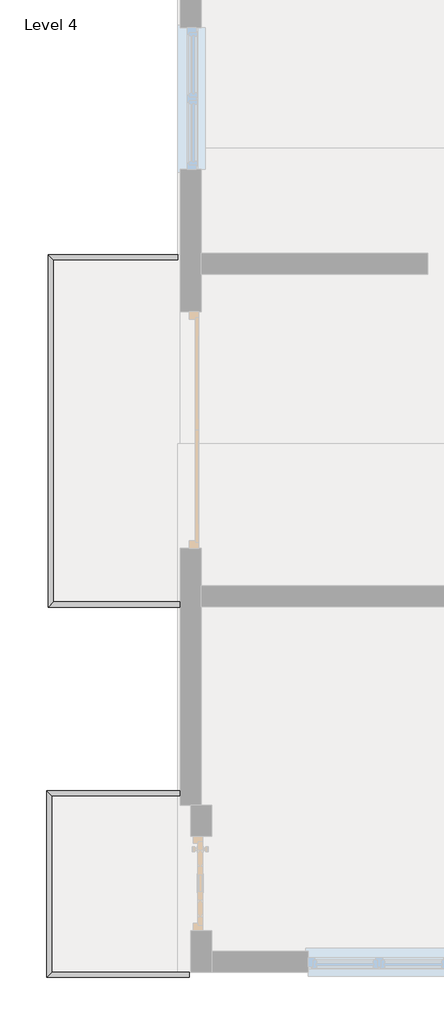
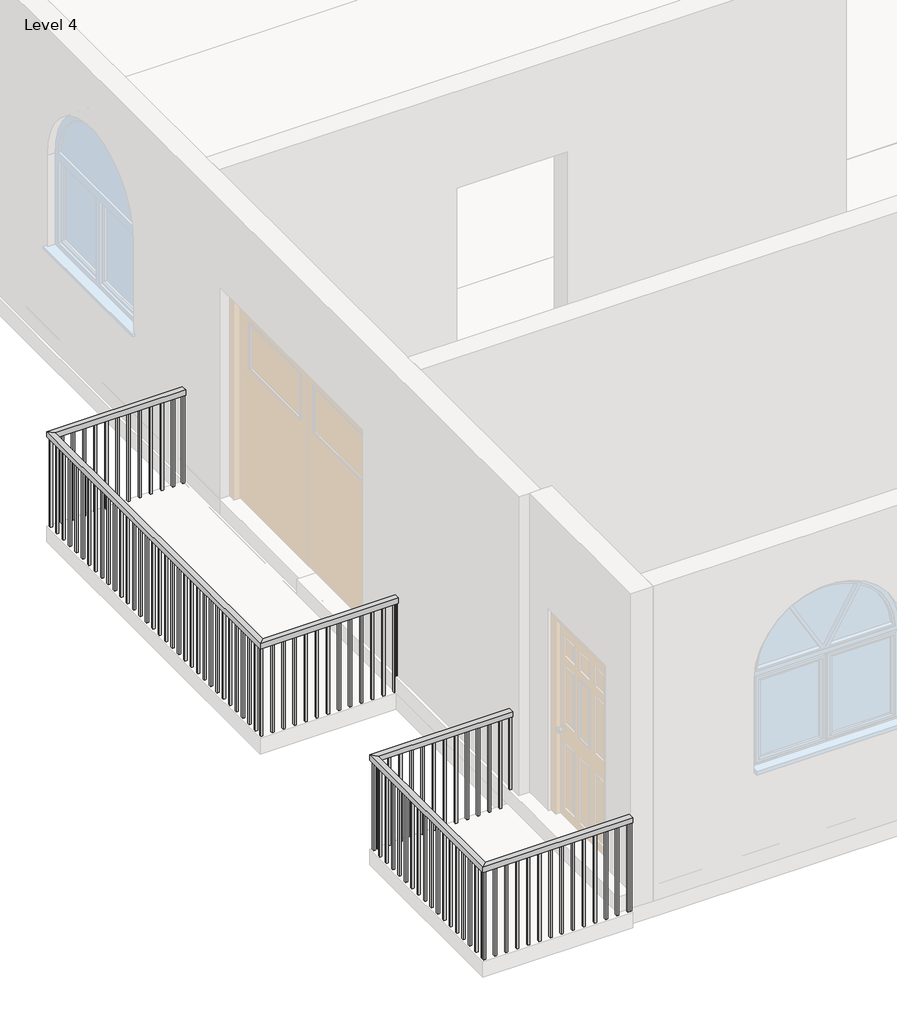
# One storey, part 3 of 7: 2 railings.
"""IFC4 building model written with IfcOpenShell, lengths in millimetres."""

from ifc_helpers import new_model, si_unit, frame, origin, place, context, project, spatial, polyline, outline, extrude, faceted_brep, element, save

model = new_model("IFC4")

# Units and contexts
model_context = context("Model", 3, world=origin())
ifc_project = project(units=[si_unit("LENGTHUNIT", "METRE", prefix="MILLI")], contexts=[model_context])

# Site, building, storey
site = spatial("IfcSite", under=ifc_project)
building = spatial("IfcBuilding", under=site)
storey = spatial("IfcBuildingStorey", under=building, Name="Level 4", Elevation=9144.0)

# Railings
placement = place(None, origin())
element("IfcRailing", 1, ObjectType="Handrail - Rectangular", at=placement, inside=storey, context=model_context, shape_type="SolidModel", body=[
    faceted_brep([(-6354.2109037, -3767.6037749, 10058.4), (-6354.2109037, -3767.6037749, 10007.6), (-6354.2109037, -3716.8037749, 10007.6), (-6354.2109037, -3716.8037749, 10058.4), (-7548.0109037, -3767.6037749, 10058.4), (-7548.0109037, -3767.6037749, 10007.6), (-7598.8109037, -3716.8037749, 10007.6), (-7598.8109037, -3716.8037749, 10058.4), (-7548.0109037, -7054.4894702, 10058.4), (-7548.0109037, -7054.4894702, 10007.6), (-7598.8109037, -7105.2894702, 10007.6), (-7598.8109037, -7105.2894702, 10058.4), (-6330.8013636, -7054.4894702, 10058.4), (-6330.8013636, -7105.2894702, 10058.4), (-6330.8013636, -7105.2894702, 10007.6), (-6330.8013636, -7054.4894702, 10007.6)], [[[0, 1, 2, 3]], [[1, 0, 4, 5]], [[2, 1, 5, 6]], [[3, 2, 6, 7]], [[0, 3, 7, 4]], [[5, 4, 8, 9]], [[6, 5, 9, 10]], [[7, 6, 10, 11]], [[4, 7, 11, 8]], [[12, 13, 14, 15]], [[9, 8, 12, 15]], [[10, 9, 15, 14]], [[11, 10, 14, 13]], [[8, 11, 13, 12]]]),
    extrude(outline(polyline([(-6363.7359037, -7089.4144702), (-6363.7359037, -7070.3644702), (-6344.6859037, -7070.3644702), (-6344.6859037, -7089.4144702), (-6363.7359037, -7089.4144702)])), frame((0.0, 0.0, 9144.0), z_axis=(0.0, 0.0, 1.0), x_axis=(1.0, 0.0, 0.0)), (0.0, 0.0, 1.0), 863.6),
    extrude(outline(polyline([(-6465.3359037, -7089.4144702), (-6465.3359037, -7070.3644702), (-6446.2859037, -7070.3644702), (-6446.2859037, -7089.4144702), (-6465.3359037, -7089.4144702)])), frame((0.0, 0.0, 9144.0), z_axis=(0.0, 0.0, 1.0), x_axis=(1.0, 0.0, 0.0)), (0.0, 0.0, 1.0), 863.6),
    extrude(outline(polyline([(-6566.9359037, -7089.4144702), (-6566.9359037, -7070.3644702), (-6547.8859037, -7070.3644702), (-6547.8859037, -7089.4144702), (-6566.9359037, -7089.4144702)])), frame((0.0, 0.0, 9144.0), z_axis=(0.0, 0.0, 1.0), x_axis=(1.0, 0.0, 0.0)), (0.0, 0.0, 1.0), 863.6),
    extrude(outline(polyline([(-6668.5359037, -7089.4144702), (-6668.5359037, -7070.3644702), (-6649.4859037, -7070.3644702), (-6649.4859037, -7089.4144702), (-6668.5359037, -7089.4144702)])), frame((0.0, 0.0, 9144.0), z_axis=(0.0, 0.0, 1.0), x_axis=(1.0, 0.0, 0.0)), (0.0, 0.0, 1.0), 863.6),
    extrude(outline(polyline([(-6770.1359037, -7089.4144702), (-6770.1359037, -7070.3644702), (-6751.0859037, -7070.3644702), (-6751.0859037, -7089.4144702), (-6770.1359037, -7089.4144702)])), frame((0.0, 0.0, 9144.0), z_axis=(0.0, 0.0, 1.0), x_axis=(1.0, 0.0, 0.0)), (0.0, 0.0, 1.0), 863.6),
    extrude(outline(polyline([(-6871.7359037, -7089.4144702), (-6871.7359037, -7070.3644702), (-6852.6859037, -7070.3644702), (-6852.6859037, -7089.4144702), (-6871.7359037, -7089.4144702)])), frame((0.0, 0.0, 9144.0), z_axis=(0.0, 0.0, 1.0), x_axis=(1.0, 0.0, 0.0)), (0.0, 0.0, 1.0), 863.6),
    extrude(outline(polyline([(-6973.3359037, -7089.4144702), (-6973.3359037, -7070.3644702), (-6954.2859037, -7070.3644702), (-6954.2859037, -7089.4144702), (-6973.3359037, -7089.4144702)])), frame((0.0, 0.0, 9144.0), z_axis=(0.0, 0.0, 1.0), x_axis=(1.0, 0.0, 0.0)), (0.0, 0.0, 1.0), 863.6),
    extrude(outline(polyline([(-7074.9359037, -7089.4144702), (-7074.9359037, -7070.3644702), (-7055.8859037, -7070.3644702), (-7055.8859037, -7089.4144702), (-7074.9359037, -7089.4144702)])), frame((0.0, 0.0, 9144.0), z_axis=(0.0, 0.0, 1.0), x_axis=(1.0, 0.0, 0.0)), (0.0, 0.0, 1.0), 863.6),
    extrude(outline(polyline([(-7176.5359037, -7089.4144702), (-7176.5359037, -7070.3644702), (-7157.4859037, -7070.3644702), (-7157.4859037, -7089.4144702), (-7176.5359037, -7089.4144702)])), frame((0.0, 0.0, 9144.0), z_axis=(0.0, 0.0, 1.0), x_axis=(1.0, 0.0, 0.0)), (0.0, 0.0, 1.0), 863.6),
    extrude(outline(polyline([(-7278.1359037, -7089.4144702), (-7278.1359037, -7070.3644702), (-7259.0859037, -7070.3644702), (-7259.0859037, -7089.4144702), (-7278.1359037, -7089.4144702)])), frame((0.0, 0.0, 9144.0), z_axis=(0.0, 0.0, 1.0), x_axis=(1.0, 0.0, 0.0)), (0.0, 0.0, 1.0), 863.6),
    extrude(outline(polyline([(-7379.7359037, -7089.4144702), (-7379.7359037, -7070.3644702), (-7360.6859037, -7070.3644702), (-7360.6859037, -7089.4144702), (-7379.7359037, -7089.4144702)])), frame((0.0, 0.0, 9144.0), z_axis=(0.0, 0.0, 1.0), x_axis=(1.0, 0.0, 0.0)), (0.0, 0.0, 1.0), 863.6),
    extrude(outline(polyline([(-7481.3359037, -7089.4144702), (-7481.3359037, -7070.3644702), (-7462.2859037, -7070.3644702), (-7462.2859037, -7089.4144702), (-7481.3359037, -7089.4144702)])), frame((0.0, 0.0, 9144.0), z_axis=(0.0, 0.0, 1.0), x_axis=(1.0, 0.0, 0.0)), (0.0, 0.0, 1.0), 863.6),
    extrude(outline(polyline([(-7582.9359037, -6983.8787749), (-7563.8859037, -6983.8787749), (-7563.8859037, -7002.9287749), (-7582.9359037, -7002.9287749), (-7582.9359037, -6983.8787749)])), frame((0.0, 0.0, 9144.0), z_axis=(0.0, 0.0, 1.0), x_axis=(1.0, 0.0, 0.0)), (0.0, 0.0, 1.0), 863.6),
    extrude(outline(polyline([(-7582.9359037, -6882.2787749), (-7563.8859037, -6882.2787749), (-7563.8859037, -6901.3287749), (-7582.9359037, -6901.3287749), (-7582.9359037, -6882.2787749)])), frame((0.0, 0.0, 9144.0), z_axis=(0.0, 0.0, 1.0), x_axis=(1.0, 0.0, 0.0)), (0.0, 0.0, 1.0), 863.6),
    extrude(outline(polyline([(-7582.9359037, -6780.6787749), (-7563.8859037, -6780.6787749), (-7563.8859037, -6799.7287749), (-7582.9359037, -6799.7287749), (-7582.9359037, -6780.6787749)])), frame((0.0, 0.0, 9144.0), z_axis=(0.0, 0.0, 1.0), x_axis=(1.0, 0.0, 0.0)), (0.0, 0.0, 1.0), 863.6),
    extrude(outline(polyline([(-7582.9359037, -6679.0787749), (-7563.8859037, -6679.0787749), (-7563.8859037, -6698.1287749), (-7582.9359037, -6698.1287749), (-7582.9359037, -6679.0787749)])), frame((0.0, 0.0, 9144.0), z_axis=(0.0, 0.0, 1.0), x_axis=(1.0, 0.0, 0.0)), (0.0, 0.0, 1.0), 863.6),
    extrude(outline(polyline([(-7582.9359037, -6577.4787749), (-7563.8859037, -6577.4787749), (-7563.8859037, -6596.5287749), (-7582.9359037, -6596.5287749), (-7582.9359037, -6577.4787749)])), frame((0.0, 0.0, 9144.0), z_axis=(0.0, 0.0, 1.0), x_axis=(1.0, 0.0, 0.0)), (0.0, 0.0, 1.0), 863.6),
    extrude(outline(polyline([(-7582.9359037, -6475.8787749), (-7563.8859037, -6475.8787749), (-7563.8859037, -6494.9287749), (-7582.9359037, -6494.9287749), (-7582.9359037, -6475.8787749)])), frame((0.0, 0.0, 9144.0), z_axis=(0.0, 0.0, 1.0), x_axis=(1.0, 0.0, 0.0)), (0.0, 0.0, 1.0), 863.6),
    extrude(outline(polyline([(-7582.9359037, -6374.2787749), (-7563.8859037, -6374.2787749), (-7563.8859037, -6393.3287749), (-7582.9359037, -6393.3287749), (-7582.9359037, -6374.2787749)])), frame((0.0, 0.0, 9144.0), z_axis=(0.0, 0.0, 1.0), x_axis=(1.0, 0.0, 0.0)), (0.0, 0.0, 1.0), 863.6),
    extrude(outline(polyline([(-7582.9359037, -6272.6787749), (-7563.8859037, -6272.6787749), (-7563.8859037, -6291.7287749), (-7582.9359037, -6291.7287749), (-7582.9359037, -6272.6787749)])), frame((0.0, 0.0, 9144.0), z_axis=(0.0, 0.0, 1.0), x_axis=(1.0, 0.0, 0.0)), (0.0, 0.0, 1.0), 863.6),
    extrude(outline(polyline([(-7582.9359037, -6171.0787749), (-7563.8859037, -6171.0787749), (-7563.8859037, -6190.1287749), (-7582.9359037, -6190.1287749), (-7582.9359037, -6171.0787749)])), frame((0.0, 0.0, 9144.0), z_axis=(0.0, 0.0, 1.0), x_axis=(1.0, 0.0, 0.0)), (0.0, 0.0, 1.0), 863.6),
    extrude(outline(polyline([(-7582.9359037, -6069.4787749), (-7563.8859037, -6069.4787749), (-7563.8859037, -6088.5287749), (-7582.9359037, -6088.5287749), (-7582.9359037, -6069.4787749)])), frame((0.0, 0.0, 9144.0), z_axis=(0.0, 0.0, 1.0), x_axis=(1.0, 0.0, 0.0)), (0.0, 0.0, 1.0), 863.6),
    extrude(outline(polyline([(-7582.9359037, -5967.8787749), (-7563.8859037, -5967.8787749), (-7563.8859037, -5986.9287749), (-7582.9359037, -5986.9287749), (-7582.9359037, -5967.8787749)])), frame((0.0, 0.0, 9144.0), z_axis=(0.0, 0.0, 1.0), x_axis=(1.0, 0.0, 0.0)), (0.0, 0.0, 1.0), 863.6),
    extrude(outline(polyline([(-7582.9359037, -5866.2787749), (-7563.8859037, -5866.2787749), (-7563.8859037, -5885.3287749), (-7582.9359037, -5885.3287749), (-7582.9359037, -5866.2787749)])), frame((0.0, 0.0, 9144.0), z_axis=(0.0, 0.0, 1.0), x_axis=(1.0, 0.0, 0.0)), (0.0, 0.0, 1.0), 863.6),
    extrude(outline(polyline([(-7582.9359037, -5764.6787749), (-7563.8859037, -5764.6787749), (-7563.8859037, -5783.7287749), (-7582.9359037, -5783.7287749), (-7582.9359037, -5764.6787749)])), frame((0.0, 0.0, 9144.0), z_axis=(0.0, 0.0, 1.0), x_axis=(1.0, 0.0, 0.0)), (0.0, 0.0, 1.0), 863.6),
    extrude(outline(polyline([(-7582.9359037, -5663.0787749), (-7563.8859037, -5663.0787749), (-7563.8859037, -5682.1287749), (-7582.9359037, -5682.1287749), (-7582.9359037, -5663.0787749)])), frame((0.0, 0.0, 9144.0), z_axis=(0.0, 0.0, 1.0), x_axis=(1.0, 0.0, 0.0)), (0.0, 0.0, 1.0), 863.6),
    extrude(outline(polyline([(-7582.9359037, -5561.4787749), (-7563.8859037, -5561.4787749), (-7563.8859037, -5580.5287749), (-7582.9359037, -5580.5287749), (-7582.9359037, -5561.4787749)])), frame((0.0, 0.0, 9144.0), z_axis=(0.0, 0.0, 1.0), x_axis=(1.0, 0.0, 0.0)), (0.0, 0.0, 1.0), 863.6),
    extrude(outline(polyline([(-7582.9359037, -5459.8787749), (-7563.8859037, -5459.8787749), (-7563.8859037, -5478.9287749), (-7582.9359037, -5478.9287749), (-7582.9359037, -5459.8787749)])), frame((0.0, 0.0, 9144.0), z_axis=(0.0, 0.0, 1.0), x_axis=(1.0, 0.0, 0.0)), (0.0, 0.0, 1.0), 863.6),
    extrude(outline(polyline([(-7582.9359037, -5358.2787749), (-7563.8859037, -5358.2787749), (-7563.8859037, -5377.3287749), (-7582.9359037, -5377.3287749), (-7582.9359037, -5358.2787749)])), frame((0.0, 0.0, 9144.0), z_axis=(0.0, 0.0, 1.0), x_axis=(1.0, 0.0, 0.0)), (0.0, 0.0, 1.0), 863.6),
    extrude(outline(polyline([(-7582.9359037, -5256.6787749), (-7563.8859037, -5256.6787749), (-7563.8859037, -5275.7287749), (-7582.9359037, -5275.7287749), (-7582.9359037, -5256.6787749)])), frame((0.0, 0.0, 9144.0), z_axis=(0.0, 0.0, 1.0), x_axis=(1.0, 0.0, 0.0)), (0.0, 0.0, 1.0), 863.6),
    extrude(outline(polyline([(-7582.9359037, -5155.0787749), (-7563.8859037, -5155.0787749), (-7563.8859037, -5174.1287749), (-7582.9359037, -5174.1287749), (-7582.9359037, -5155.0787749)])), frame((0.0, 0.0, 9144.0), z_axis=(0.0, 0.0, 1.0), x_axis=(1.0, 0.0, 0.0)), (0.0, 0.0, 1.0), 863.6),
    extrude(outline(polyline([(-7582.9359037, -5053.4787749), (-7563.8859037, -5053.4787749), (-7563.8859037, -5072.5287749), (-7582.9359037, -5072.5287749), (-7582.9359037, -5053.4787749)])), frame((0.0, 0.0, 9144.0), z_axis=(0.0, 0.0, 1.0), x_axis=(1.0, 0.0, 0.0)), (0.0, 0.0, 1.0), 863.6),
    extrude(outline(polyline([(-7582.9359037, -4951.8787749), (-7563.8859037, -4951.8787749), (-7563.8859037, -4970.9287749), (-7582.9359037, -4970.9287749), (-7582.9359037, -4951.8787749)])), frame((0.0, 0.0, 9144.0), z_axis=(0.0, 0.0, 1.0), x_axis=(1.0, 0.0, 0.0)), (0.0, 0.0, 1.0), 863.6),
    extrude(outline(polyline([(-7582.9359037, -4850.2787749), (-7563.8859037, -4850.2787749), (-7563.8859037, -4869.3287749), (-7582.9359037, -4869.3287749), (-7582.9359037, -4850.2787749)])), frame((0.0, 0.0, 9144.0), z_axis=(0.0, 0.0, 1.0), x_axis=(1.0, 0.0, 0.0)), (0.0, 0.0, 1.0), 863.6),
    extrude(outline(polyline([(-7582.9359037, -4748.6787749), (-7563.8859037, -4748.6787749), (-7563.8859037, -4767.7287749), (-7582.9359037, -4767.7287749), (-7582.9359037, -4748.6787749)])), frame((0.0, 0.0, 9144.0), z_axis=(0.0, 0.0, 1.0), x_axis=(1.0, 0.0, 0.0)), (0.0, 0.0, 1.0), 863.6),
    extrude(outline(polyline([(-7582.9359037, -4647.0787749), (-7563.8859037, -4647.0787749), (-7563.8859037, -4666.1287749), (-7582.9359037, -4666.1287749), (-7582.9359037, -4647.0787749)])), frame((0.0, 0.0, 9144.0), z_axis=(0.0, 0.0, 1.0), x_axis=(1.0, 0.0, 0.0)), (0.0, 0.0, 1.0), 863.6),
    extrude(outline(polyline([(-7582.9359037, -4545.4787749), (-7563.8859037, -4545.4787749), (-7563.8859037, -4564.5287749), (-7582.9359037, -4564.5287749), (-7582.9359037, -4545.4787749)])), frame((0.0, 0.0, 9144.0), z_axis=(0.0, 0.0, 1.0), x_axis=(1.0, 0.0, 0.0)), (0.0, 0.0, 1.0), 863.6),
    extrude(outline(polyline([(-7582.9359037, -4443.8787749), (-7563.8859037, -4443.8787749), (-7563.8859037, -4462.9287749), (-7582.9359037, -4462.9287749), (-7582.9359037, -4443.8787749)])), frame((0.0, 0.0, 9144.0), z_axis=(0.0, 0.0, 1.0), x_axis=(1.0, 0.0, 0.0)), (0.0, 0.0, 1.0), 863.6),
    extrude(outline(polyline([(-7582.9359037, -4342.2787749), (-7563.8859037, -4342.2787749), (-7563.8859037, -4361.3287749), (-7582.9359037, -4361.3287749), (-7582.9359037, -4342.2787749)])), frame((0.0, 0.0, 9144.0), z_axis=(0.0, 0.0, 1.0), x_axis=(1.0, 0.0, 0.0)), (0.0, 0.0, 1.0), 863.6),
    extrude(outline(polyline([(-7582.9359037, -4240.6787749), (-7563.8859037, -4240.6787749), (-7563.8859037, -4259.7287749), (-7582.9359037, -4259.7287749), (-7582.9359037, -4240.6787749)])), frame((0.0, 0.0, 9144.0), z_axis=(0.0, 0.0, 1.0), x_axis=(1.0, 0.0, 0.0)), (0.0, 0.0, 1.0), 863.6),
    extrude(outline(polyline([(-7582.9359037, -4139.0787749), (-7563.8859037, -4139.0787749), (-7563.8859037, -4158.1287749), (-7582.9359037, -4158.1287749), (-7582.9359037, -4139.0787749)])), frame((0.0, 0.0, 9144.0), z_axis=(0.0, 0.0, 1.0), x_axis=(1.0, 0.0, 0.0)), (0.0, 0.0, 1.0), 863.6),
    extrude(outline(polyline([(-7582.9359037, -4037.4787749), (-7563.8859037, -4037.4787749), (-7563.8859037, -4056.5287749), (-7582.9359037, -4056.5287749), (-7582.9359037, -4037.4787749)])), frame((0.0, 0.0, 9144.0), z_axis=(0.0, 0.0, 1.0), x_axis=(1.0, 0.0, 0.0)), (0.0, 0.0, 1.0), 863.6),
    extrude(outline(polyline([(-7582.9359037, -3935.8787749), (-7563.8859037, -3935.8787749), (-7563.8859037, -3954.9287749), (-7582.9359037, -3954.9287749), (-7582.9359037, -3935.8787749)])), frame((0.0, 0.0, 9144.0), z_axis=(0.0, 0.0, 1.0), x_axis=(1.0, 0.0, 0.0)), (0.0, 0.0, 1.0), 863.6),
    extrude(outline(polyline([(-7582.9359037, -3834.2787749), (-7563.8859037, -3834.2787749), (-7563.8859037, -3853.3287749), (-7582.9359037, -3853.3287749), (-7582.9359037, -3834.2787749)])), frame((0.0, 0.0, 9144.0), z_axis=(0.0, 0.0, 1.0), x_axis=(1.0, 0.0, 0.0)), (0.0, 0.0, 1.0), 863.6),
    extrude(outline(polyline([(-7462.2859037, -3732.6787749), (-7462.2859037, -3751.7287749), (-7481.3359037, -3751.7287749), (-7481.3359037, -3732.6787749), (-7462.2859037, -3732.6787749)])), frame((0.0, 0.0, 9144.0), z_axis=(0.0, 0.0, 1.0), x_axis=(1.0, 0.0, 0.0)), (0.0, 0.0, 1.0), 863.6),
    extrude(outline(polyline([(-7360.6859037, -3732.6787749), (-7360.6859037, -3751.7287749), (-7379.7359037, -3751.7287749), (-7379.7359037, -3732.6787749), (-7360.6859037, -3732.6787749)])), frame((0.0, 0.0, 9144.0), z_axis=(0.0, 0.0, 1.0), x_axis=(1.0, 0.0, 0.0)), (0.0, 0.0, 1.0), 863.6),
    extrude(outline(polyline([(-7259.0859037, -3732.6787749), (-7259.0859037, -3751.7287749), (-7278.1359037, -3751.7287749), (-7278.1359037, -3732.6787749), (-7259.0859037, -3732.6787749)])), frame((0.0, 0.0, 9144.0), z_axis=(0.0, 0.0, 1.0), x_axis=(1.0, 0.0, 0.0)), (0.0, 0.0, 1.0), 863.6),
    extrude(outline(polyline([(-7157.4859037, -3732.6787749), (-7157.4859037, -3751.7287749), (-7176.5359037, -3751.7287749), (-7176.5359037, -3732.6787749), (-7157.4859037, -3732.6787749)])), frame((0.0, 0.0, 9144.0), z_axis=(0.0, 0.0, 1.0), x_axis=(1.0, 0.0, 0.0)), (0.0, 0.0, 1.0), 863.6),
    extrude(outline(polyline([(-7055.8859037, -3732.6787749), (-7055.8859037, -3751.7287749), (-7074.9359037, -3751.7287749), (-7074.9359037, -3732.6787749), (-7055.8859037, -3732.6787749)])), frame((0.0, 0.0, 9144.0), z_axis=(0.0, 0.0, 1.0), x_axis=(1.0, 0.0, 0.0)), (0.0, 0.0, 1.0), 863.6),
    extrude(outline(polyline([(-6954.2859037, -3732.6787749), (-6954.2859037, -3751.7287749), (-6973.3359037, -3751.7287749), (-6973.3359037, -3732.6787749), (-6954.2859037, -3732.6787749)])), frame((0.0, 0.0, 9144.0), z_axis=(0.0, 0.0, 1.0), x_axis=(1.0, 0.0, 0.0)), (0.0, 0.0, 1.0), 863.6),
    extrude(outline(polyline([(-6852.6859037, -3732.6787749), (-6852.6859037, -3751.7287749), (-6871.7359037, -3751.7287749), (-6871.7359037, -3732.6787749), (-6852.6859037, -3732.6787749)])), frame((0.0, 0.0, 9144.0), z_axis=(0.0, 0.0, 1.0), x_axis=(1.0, 0.0, 0.0)), (0.0, 0.0, 1.0), 863.6),
    extrude(outline(polyline([(-6751.0859037, -3732.6787749), (-6751.0859037, -3751.7287749), (-6770.1359037, -3751.7287749), (-6770.1359037, -3732.6787749), (-6751.0859037, -3732.6787749)])), frame((0.0, 0.0, 9144.0), z_axis=(0.0, 0.0, 1.0), x_axis=(1.0, 0.0, 0.0)), (0.0, 0.0, 1.0), 863.6),
    extrude(outline(polyline([(-6649.4859037, -3732.6787749), (-6649.4859037, -3751.7287749), (-6668.5359037, -3751.7287749), (-6668.5359037, -3732.6787749), (-6649.4859037, -3732.6787749)])), frame((0.0, 0.0, 9144.0), z_axis=(0.0, 0.0, 1.0), x_axis=(1.0, 0.0, 0.0)), (0.0, 0.0, 1.0), 863.6),
    extrude(outline(polyline([(-6547.8859037, -3732.6787749), (-6547.8859037, -3751.7287749), (-6566.9359037, -3751.7287749), (-6566.9359037, -3732.6787749), (-6547.8859037, -3732.6787749)])), frame((0.0, 0.0, 9144.0), z_axis=(0.0, 0.0, 1.0), x_axis=(1.0, 0.0, 0.0)), (0.0, 0.0, 1.0), 863.6),
    extrude(outline(polyline([(-6446.2859037, -3732.6787749), (-6446.2859037, -3751.7287749), (-6465.3359037, -3751.7287749), (-6465.3359037, -3732.6787749), (-6446.2859037, -3732.6787749)])), frame((0.0, 0.0, 9144.0), z_axis=(0.0, 0.0, 1.0), x_axis=(1.0, 0.0, 0.0)), (0.0, 0.0, 1.0), 863.6),
    extrude(outline(polyline([(-7582.9359037, -7070.3644702), (-7563.8859037, -7070.3644702), (-7563.8859037, -7089.4144702), (-7582.9359037, -7089.4144702), (-7582.9359037, -7070.3644702)])), frame((0.0, 0.0, 9144.0), z_axis=(0.0, 0.0, 1.0), x_axis=(1.0, 0.0, 0.0)), (0.0, 0.0, 1.0), 863.6),
    extrude(outline(polyline([(-7563.8859037, -3732.6787749), (-7563.8859037, -3751.7287749), (-7582.9359037, -3751.7287749), (-7582.9359037, -3732.6787749), (-7563.8859037, -3732.6787749)])), frame((0.0, 0.0, 9144.0), z_axis=(0.0, 0.0, 1.0), x_axis=(1.0, 0.0, 0.0)), (0.0, 0.0, 1.0), 863.6),
    extrude(outline(polyline([(-6349.8513636, -7089.4144702), (-6349.8513636, -7070.3644702), (-6330.8013636, -7070.3644702), (-6330.8013636, -7089.4144702), (-6349.8513636, -7089.4144702)])), frame((0.0, 0.0, 9144.0), z_axis=(0.0, 0.0, 1.0), x_axis=(1.0, 0.0, 0.0)), (0.0, 0.0, 1.0), 863.6),
    extrude(outline(polyline([(-6354.2109037, -3732.6787749), (-6354.2109037, -3751.7287749), (-6373.2609037, -3751.7287749), (-6373.2609037, -3732.6787749), (-6354.2109037, -3732.6787749)])), frame((0.0, 0.0, 9144.0), z_axis=(0.0, 0.0, 1.0), x_axis=(1.0, 0.0, 0.0)), (0.0, 0.0, 1.0), 863.6),
])
element("IfcRailing", 2, ObjectType="Handrail - Rectangular", at=placement, inside=storey, context=model_context, shape_type="SolidModel", body=[
    faceted_brep([(-6330.8013636, -8918.8845215, 10058.4), (-6330.8013636, -8918.8845215, 10007.6), (-6330.8013636, -8868.0845215, 10007.6), (-6330.8013636, -8868.0845215, 10058.4), (-7563.8859037, -8918.8845215, 10058.4), (-7563.8859037, -8918.8845215, 10007.6), (-7614.6859037, -8868.0845215, 10007.6), (-7614.6859037, -8868.0845215, 10058.4), (-7563.8859037, -10612.9037749, 10058.4), (-7563.8859037, -10612.9037749, 10007.6), (-7614.6859037, -10663.7037749, 10007.6), (-7614.6859037, -10663.7037749, 10058.4), (-6243.0859037, -10612.9037749, 10058.4), (-6243.0859037, -10663.7037749, 10058.4), (-6243.0859037, -10663.7037749, 10007.6), (-6243.0859037, -10612.9037749, 10007.6)], [[[0, 1, 2, 3]], [[1, 0, 4, 5]], [[2, 1, 5, 6]], [[3, 2, 6, 7]], [[0, 3, 7, 4]], [[5, 4, 8, 9]], [[6, 5, 9, 10]], [[7, 6, 10, 11]], [[4, 7, 11, 8]], [[12, 13, 14, 15]], [[9, 8, 12, 15]], [[10, 9, 15, 14]], [[11, 10, 14, 13]], [[8, 11, 13, 12]]]),
    extrude(outline(polyline([(-6278.0109037, -10647.8287749), (-6278.0109037, -10628.7787749), (-6258.9609037, -10628.7787749), (-6258.9609037, -10647.8287749), (-6278.0109037, -10647.8287749)])), frame((0.0, 0.0, 9144.0), z_axis=(0.0, 0.0, 1.0), x_axis=(1.0, 0.0, 0.0)), (0.0, 0.0, 1.0), 863.6),
    extrude(outline(polyline([(-6379.6109037, -10647.8287749), (-6379.6109037, -10628.7787749), (-6360.5609037, -10628.7787749), (-6360.5609037, -10647.8287749), (-6379.6109037, -10647.8287749)])), frame((0.0, 0.0, 9144.0), z_axis=(0.0, 0.0, 1.0), x_axis=(1.0, 0.0, 0.0)), (0.0, 0.0, 1.0), 863.6),
    extrude(outline(polyline([(-6481.2109037, -10647.8287749), (-6481.2109037, -10628.7787749), (-6462.1609037, -10628.7787749), (-6462.1609037, -10647.8287749), (-6481.2109037, -10647.8287749)])), frame((0.0, 0.0, 9144.0), z_axis=(0.0, 0.0, 1.0), x_axis=(1.0, 0.0, 0.0)), (0.0, 0.0, 1.0), 863.6),
    extrude(outline(polyline([(-6582.8109037, -10647.8287749), (-6582.8109037, -10628.7787749), (-6563.7609037, -10628.7787749), (-6563.7609037, -10647.8287749), (-6582.8109037, -10647.8287749)])), frame((0.0, 0.0, 9144.0), z_axis=(0.0, 0.0, 1.0), x_axis=(1.0, 0.0, 0.0)), (0.0, 0.0, 1.0), 863.6),
    extrude(outline(polyline([(-6684.4109037, -10647.8287749), (-6684.4109037, -10628.7787749), (-6665.3609037, -10628.7787749), (-6665.3609037, -10647.8287749), (-6684.4109037, -10647.8287749)])), frame((0.0, 0.0, 9144.0), z_axis=(0.0, 0.0, 1.0), x_axis=(1.0, 0.0, 0.0)), (0.0, 0.0, 1.0), 863.6),
    extrude(outline(polyline([(-6786.0109037, -10647.8287749), (-6786.0109037, -10628.7787749), (-6766.9609037, -10628.7787749), (-6766.9609037, -10647.8287749), (-6786.0109037, -10647.8287749)])), frame((0.0, 0.0, 9144.0), z_axis=(0.0, 0.0, 1.0), x_axis=(1.0, 0.0, 0.0)), (0.0, 0.0, 1.0), 863.6),
    extrude(outline(polyline([(-6887.6109037, -10647.8287749), (-6887.6109037, -10628.7787749), (-6868.5609037, -10628.7787749), (-6868.5609037, -10647.8287749), (-6887.6109037, -10647.8287749)])), frame((0.0, 0.0, 9144.0), z_axis=(0.0, 0.0, 1.0), x_axis=(1.0, 0.0, 0.0)), (0.0, 0.0, 1.0), 863.6),
    extrude(outline(polyline([(-6989.2109037, -10647.8287749), (-6989.2109037, -10628.7787749), (-6970.1609037, -10628.7787749), (-6970.1609037, -10647.8287749), (-6989.2109037, -10647.8287749)])), frame((0.0, 0.0, 9144.0), z_axis=(0.0, 0.0, 1.0), x_axis=(1.0, 0.0, 0.0)), (0.0, 0.0, 1.0), 863.6),
    extrude(outline(polyline([(-7090.8109037, -10647.8287749), (-7090.8109037, -10628.7787749), (-7071.7609037, -10628.7787749), (-7071.7609037, -10647.8287749), (-7090.8109037, -10647.8287749)])), frame((0.0, 0.0, 9144.0), z_axis=(0.0, 0.0, 1.0), x_axis=(1.0, 0.0, 0.0)), (0.0, 0.0, 1.0), 863.6),
    extrude(outline(polyline([(-7192.4109037, -10647.8287749), (-7192.4109037, -10628.7787749), (-7173.3609037, -10628.7787749), (-7173.3609037, -10647.8287749), (-7192.4109037, -10647.8287749)])), frame((0.0, 0.0, 9144.0), z_axis=(0.0, 0.0, 1.0), x_axis=(1.0, 0.0, 0.0)), (0.0, 0.0, 1.0), 863.6),
    extrude(outline(polyline([(-7294.0109037, -10647.8287749), (-7294.0109037, -10628.7787749), (-7274.9609037, -10628.7787749), (-7274.9609037, -10647.8287749), (-7294.0109037, -10647.8287749)])), frame((0.0, 0.0, 9144.0), z_axis=(0.0, 0.0, 1.0), x_axis=(1.0, 0.0, 0.0)), (0.0, 0.0, 1.0), 863.6),
    extrude(outline(polyline([(-7395.6109037, -10647.8287749), (-7395.6109037, -10628.7787749), (-7376.5609037, -10628.7787749), (-7376.5609037, -10647.8287749), (-7395.6109037, -10647.8287749)])), frame((0.0, 0.0, 9144.0), z_axis=(0.0, 0.0, 1.0), x_axis=(1.0, 0.0, 0.0)), (0.0, 0.0, 1.0), 863.6),
    extrude(outline(polyline([(-7497.2109037, -10647.8287749), (-7497.2109037, -10628.7787749), (-7478.1609037, -10628.7787749), (-7478.1609037, -10647.8287749), (-7497.2109037, -10647.8287749)])), frame((0.0, 0.0, 9144.0), z_axis=(0.0, 0.0, 1.0), x_axis=(1.0, 0.0, 0.0)), (0.0, 0.0, 1.0), 863.6),
    extrude(outline(polyline([(-7598.8109037, -10611.1595215), (-7579.7609037, -10611.1595215), (-7579.7609037, -10630.2095215), (-7598.8109037, -10630.2095215), (-7598.8109037, -10611.1595215)])), frame((0.0, 0.0, 9144.0), z_axis=(0.0, 0.0, 1.0), x_axis=(1.0, 0.0, 0.0)), (0.0, 0.0, 1.0), 863.6),
    extrude(outline(polyline([(-7598.8109037, -10509.5595215), (-7579.7609037, -10509.5595215), (-7579.7609037, -10528.6095215), (-7598.8109037, -10528.6095215), (-7598.8109037, -10509.5595215)])), frame((0.0, 0.0, 9144.0), z_axis=(0.0, 0.0, 1.0), x_axis=(1.0, 0.0, 0.0)), (0.0, 0.0, 1.0), 863.6),
    extrude(outline(polyline([(-7598.8109037, -10407.9595215), (-7579.7609037, -10407.9595215), (-7579.7609037, -10427.0095215), (-7598.8109037, -10427.0095215), (-7598.8109037, -10407.9595215)])), frame((0.0, 0.0, 9144.0), z_axis=(0.0, 0.0, 1.0), x_axis=(1.0, 0.0, 0.0)), (0.0, 0.0, 1.0), 863.6),
    extrude(outline(polyline([(-7598.8109037, -10306.3595215), (-7579.7609037, -10306.3595215), (-7579.7609037, -10325.4095215), (-7598.8109037, -10325.4095215), (-7598.8109037, -10306.3595215)])), frame((0.0, 0.0, 9144.0), z_axis=(0.0, 0.0, 1.0), x_axis=(1.0, 0.0, 0.0)), (0.0, 0.0, 1.0), 863.6),
    extrude(outline(polyline([(-7598.8109037, -10204.7595215), (-7579.7609037, -10204.7595215), (-7579.7609037, -10223.8095215), (-7598.8109037, -10223.8095215), (-7598.8109037, -10204.7595215)])), frame((0.0, 0.0, 9144.0), z_axis=(0.0, 0.0, 1.0), x_axis=(1.0, 0.0, 0.0)), (0.0, 0.0, 1.0), 863.6),
    extrude(outline(polyline([(-7598.8109037, -10103.1595215), (-7579.7609037, -10103.1595215), (-7579.7609037, -10122.2095215), (-7598.8109037, -10122.2095215), (-7598.8109037, -10103.1595215)])), frame((0.0, 0.0, 9144.0), z_axis=(0.0, 0.0, 1.0), x_axis=(1.0, 0.0, 0.0)), (0.0, 0.0, 1.0), 863.6),
    extrude(outline(polyline([(-7598.8109037, -10001.5595215), (-7579.7609037, -10001.5595215), (-7579.7609037, -10020.6095215), (-7598.8109037, -10020.6095215), (-7598.8109037, -10001.5595215)])), frame((0.0, 0.0, 9144.0), z_axis=(0.0, 0.0, 1.0), x_axis=(1.0, 0.0, 0.0)), (0.0, 0.0, 1.0), 863.6),
    extrude(outline(polyline([(-7598.8109037, -9899.9595215), (-7579.7609037, -9899.9595215), (-7579.7609037, -9919.0095215), (-7598.8109037, -9919.0095215), (-7598.8109037, -9899.9595215)])), frame((0.0, 0.0, 9144.0), z_axis=(0.0, 0.0, 1.0), x_axis=(1.0, 0.0, 0.0)), (0.0, 0.0, 1.0), 863.6),
    extrude(outline(polyline([(-7598.8109037, -9798.3595215), (-7579.7609037, -9798.3595215), (-7579.7609037, -9817.4095215), (-7598.8109037, -9817.4095215), (-7598.8109037, -9798.3595215)])), frame((0.0, 0.0, 9144.0), z_axis=(0.0, 0.0, 1.0), x_axis=(1.0, 0.0, 0.0)), (0.0, 0.0, 1.0), 863.6),
    extrude(outline(polyline([(-7598.8109037, -9696.7595215), (-7579.7609037, -9696.7595215), (-7579.7609037, -9715.8095215), (-7598.8109037, -9715.8095215), (-7598.8109037, -9696.7595215)])), frame((0.0, 0.0, 9144.0), z_axis=(0.0, 0.0, 1.0), x_axis=(1.0, 0.0, 0.0)), (0.0, 0.0, 1.0), 863.6),
    extrude(outline(polyline([(-7598.8109037, -9595.1595215), (-7579.7609037, -9595.1595215), (-7579.7609037, -9614.2095215), (-7598.8109037, -9614.2095215), (-7598.8109037, -9595.1595215)])), frame((0.0, 0.0, 9144.0), z_axis=(0.0, 0.0, 1.0), x_axis=(1.0, 0.0, 0.0)), (0.0, 0.0, 1.0), 863.6),
    extrude(outline(polyline([(-7598.8109037, -9493.5595215), (-7579.7609037, -9493.5595215), (-7579.7609037, -9512.6095215), (-7598.8109037, -9512.6095215), (-7598.8109037, -9493.5595215)])), frame((0.0, 0.0, 9144.0), z_axis=(0.0, 0.0, 1.0), x_axis=(1.0, 0.0, 0.0)), (0.0, 0.0, 1.0), 863.6),
    extrude(outline(polyline([(-7598.8109037, -9391.9595215), (-7579.7609037, -9391.9595215), (-7579.7609037, -9411.0095215), (-7598.8109037, -9411.0095215), (-7598.8109037, -9391.9595215)])), frame((0.0, 0.0, 9144.0), z_axis=(0.0, 0.0, 1.0), x_axis=(1.0, 0.0, 0.0)), (0.0, 0.0, 1.0), 863.6),
    extrude(outline(polyline([(-7598.8109037, -9290.3595215), (-7579.7609037, -9290.3595215), (-7579.7609037, -9309.4095215), (-7598.8109037, -9309.4095215), (-7598.8109037, -9290.3595215)])), frame((0.0, 0.0, 9144.0), z_axis=(0.0, 0.0, 1.0), x_axis=(1.0, 0.0, 0.0)), (0.0, 0.0, 1.0), 863.6),
    extrude(outline(polyline([(-7598.8109037, -9188.7595215), (-7579.7609037, -9188.7595215), (-7579.7609037, -9207.8095215), (-7598.8109037, -9207.8095215), (-7598.8109037, -9188.7595215)])), frame((0.0, 0.0, 9144.0), z_axis=(0.0, 0.0, 1.0), x_axis=(1.0, 0.0, 0.0)), (0.0, 0.0, 1.0), 863.6),
    extrude(outline(polyline([(-7598.8109037, -9087.1595215), (-7579.7609037, -9087.1595215), (-7579.7609037, -9106.2095215), (-7598.8109037, -9106.2095215), (-7598.8109037, -9087.1595215)])), frame((0.0, 0.0, 9144.0), z_axis=(0.0, 0.0, 1.0), x_axis=(1.0, 0.0, 0.0)), (0.0, 0.0, 1.0), 863.6),
    extrude(outline(polyline([(-7598.8109037, -8985.5595215), (-7579.7609037, -8985.5595215), (-7579.7609037, -9004.6095215), (-7598.8109037, -9004.6095215), (-7598.8109037, -8985.5595215)])), frame((0.0, 0.0, 9144.0), z_axis=(0.0, 0.0, 1.0), x_axis=(1.0, 0.0, 0.0)), (0.0, 0.0, 1.0), 863.6),
    extrude(outline(polyline([(-7540.4763636, -8883.9595215), (-7540.4763636, -8903.0095215), (-7559.5263636, -8903.0095215), (-7559.5263636, -8883.9595215), (-7540.4763636, -8883.9595215)])), frame((0.0, 0.0, 9144.0), z_axis=(0.0, 0.0, 1.0), x_axis=(1.0, 0.0, 0.0)), (0.0, 0.0, 1.0), 863.6),
    extrude(outline(polyline([(-7438.8763636, -8883.9595215), (-7438.8763636, -8903.0095215), (-7457.9263636, -8903.0095215), (-7457.9263636, -8883.9595215), (-7438.8763636, -8883.9595215)])), frame((0.0, 0.0, 9144.0), z_axis=(0.0, 0.0, 1.0), x_axis=(1.0, 0.0, 0.0)), (0.0, 0.0, 1.0), 863.6),
    extrude(outline(polyline([(-7337.2763636, -8883.9595215), (-7337.2763636, -8903.0095215), (-7356.3263636, -8903.0095215), (-7356.3263636, -8883.9595215), (-7337.2763636, -8883.9595215)])), frame((0.0, 0.0, 9144.0), z_axis=(0.0, 0.0, 1.0), x_axis=(1.0, 0.0, 0.0)), (0.0, 0.0, 1.0), 863.6),
    extrude(outline(polyline([(-7235.6763636, -8883.9595215), (-7235.6763636, -8903.0095215), (-7254.7263636, -8903.0095215), (-7254.7263636, -8883.9595215), (-7235.6763636, -8883.9595215)])), frame((0.0, 0.0, 9144.0), z_axis=(0.0, 0.0, 1.0), x_axis=(1.0, 0.0, 0.0)), (0.0, 0.0, 1.0), 863.6),
    extrude(outline(polyline([(-7134.0763636, -8883.9595215), (-7134.0763636, -8903.0095215), (-7153.1263636, -8903.0095215), (-7153.1263636, -8883.9595215), (-7134.0763636, -8883.9595215)])), frame((0.0, 0.0, 9144.0), z_axis=(0.0, 0.0, 1.0), x_axis=(1.0, 0.0, 0.0)), (0.0, 0.0, 1.0), 863.6),
    extrude(outline(polyline([(-7032.4763636, -8883.9595215), (-7032.4763636, -8903.0095215), (-7051.5263636, -8903.0095215), (-7051.5263636, -8883.9595215), (-7032.4763636, -8883.9595215)])), frame((0.0, 0.0, 9144.0), z_axis=(0.0, 0.0, 1.0), x_axis=(1.0, 0.0, 0.0)), (0.0, 0.0, 1.0), 863.6),
    extrude(outline(polyline([(-6930.8763636, -8883.9595215), (-6930.8763636, -8903.0095215), (-6949.9263636, -8903.0095215), (-6949.9263636, -8883.9595215), (-6930.8763636, -8883.9595215)])), frame((0.0, 0.0, 9144.0), z_axis=(0.0, 0.0, 1.0), x_axis=(1.0, 0.0, 0.0)), (0.0, 0.0, 1.0), 863.6),
    extrude(outline(polyline([(-6829.2763636, -8883.9595215), (-6829.2763636, -8903.0095215), (-6848.3263636, -8903.0095215), (-6848.3263636, -8883.9595215), (-6829.2763636, -8883.9595215)])), frame((0.0, 0.0, 9144.0), z_axis=(0.0, 0.0, 1.0), x_axis=(1.0, 0.0, 0.0)), (0.0, 0.0, 1.0), 863.6),
    extrude(outline(polyline([(-6727.6763636, -8883.9595215), (-6727.6763636, -8903.0095215), (-6746.7263636, -8903.0095215), (-6746.7263636, -8883.9595215), (-6727.6763636, -8883.9595215)])), frame((0.0, 0.0, 9144.0), z_axis=(0.0, 0.0, 1.0), x_axis=(1.0, 0.0, 0.0)), (0.0, 0.0, 1.0), 863.6),
    extrude(outline(polyline([(-6626.0763636, -8883.9595215), (-6626.0763636, -8903.0095215), (-6645.1263636, -8903.0095215), (-6645.1263636, -8883.9595215), (-6626.0763636, -8883.9595215)])), frame((0.0, 0.0, 9144.0), z_axis=(0.0, 0.0, 1.0), x_axis=(1.0, 0.0, 0.0)), (0.0, 0.0, 1.0), 863.6),
    extrude(outline(polyline([(-6524.4763636, -8883.9595215), (-6524.4763636, -8903.0095215), (-6543.5263636, -8903.0095215), (-6543.5263636, -8883.9595215), (-6524.4763636, -8883.9595215)])), frame((0.0, 0.0, 9144.0), z_axis=(0.0, 0.0, 1.0), x_axis=(1.0, 0.0, 0.0)), (0.0, 0.0, 1.0), 863.6),
    extrude(outline(polyline([(-6422.8763636, -8883.9595215), (-6422.8763636, -8903.0095215), (-6441.9263636, -8903.0095215), (-6441.9263636, -8883.9595215), (-6422.8763636, -8883.9595215)])), frame((0.0, 0.0, 9144.0), z_axis=(0.0, 0.0, 1.0), x_axis=(1.0, 0.0, 0.0)), (0.0, 0.0, 1.0), 863.6),
    extrude(outline(polyline([(-7598.8109037, -10628.7787749), (-7579.7609037, -10628.7787749), (-7579.7609037, -10647.8287749), (-7598.8109037, -10647.8287749), (-7598.8109037, -10628.7787749)])), frame((0.0, 0.0, 9144.0), z_axis=(0.0, 0.0, 1.0), x_axis=(1.0, 0.0, 0.0)), (0.0, 0.0, 1.0), 863.6),
    extrude(outline(polyline([(-7579.7609037, -8883.9595215), (-7579.7609037, -8903.0095215), (-7598.8109037, -8903.0095215), (-7598.8109037, -8883.9595215), (-7579.7609037, -8883.9595215)])), frame((0.0, 0.0, 9144.0), z_axis=(0.0, 0.0, 1.0), x_axis=(1.0, 0.0, 0.0)), (0.0, 0.0, 1.0), 863.6),
    extrude(outline(polyline([(-6262.1359037, -10647.8287749), (-6262.1359037, -10628.7787749), (-6243.0859037, -10628.7787749), (-6243.0859037, -10647.8287749), (-6262.1359037, -10647.8287749)])), frame((0.0, 0.0, 9144.0), z_axis=(0.0, 0.0, 1.0), x_axis=(1.0, 0.0, 0.0)), (0.0, 0.0, 1.0), 863.6),
    extrude(outline(polyline([(-6330.8013636, -8883.9595215), (-6330.8013636, -8903.0095215), (-6349.8513636, -8903.0095215), (-6349.8513636, -8883.9595215), (-6330.8013636, -8883.9595215)])), frame((0.0, 0.0, 9144.0), z_axis=(0.0, 0.0, 1.0), x_axis=(1.0, 0.0, 0.0)), (0.0, 0.0, 1.0), 863.6),
])

save(model, "model.ifc")

# Revit data of these elements
# Type "Handrail - Rectangular"
#   Assembly Code = "C2010400"
#   built-in parameter 1008612 = 0.0416667 (stored number, unit not read)
#   built-in parameter 1008611 = 0.0416667 (stored number, unit not read)
#   built-in parameter 1008609 = 0.333333 (stored number, unit not read)
#   built-in parameter 1008604 = 0.166667 (stored number, unit not read)
#   built-in parameter 1008603 = 0.166667 (stored number, unit not read)
#   Railing Height = 3' - 0"
#   built-in parameter 1008630 = 2
#   built-in parameter 1008610 = 2
#   built-in parameter 1008618 = Baluster - Square : 3/4"
# Elements 1, 2 (IfcRailing, "Handrail - Rectangular")
#   Phase Created = New Construction
